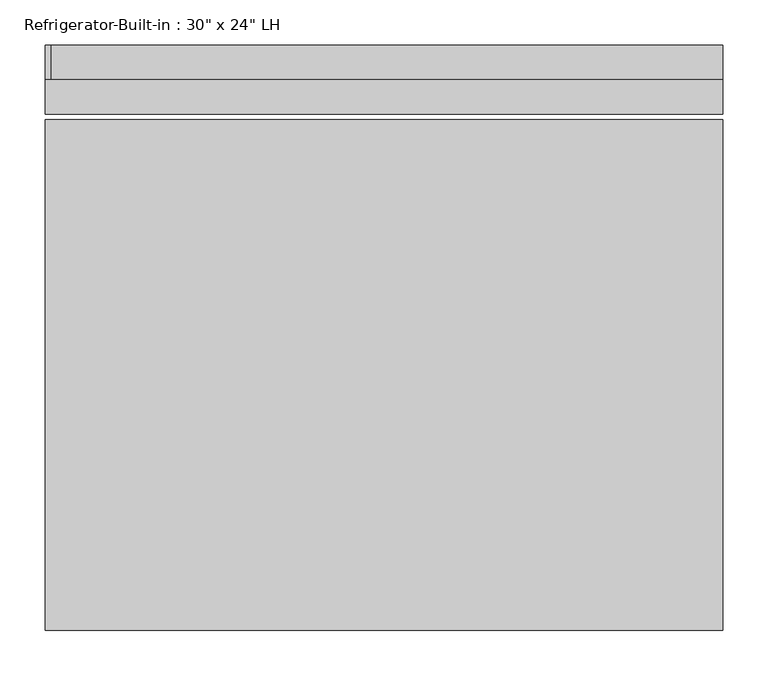
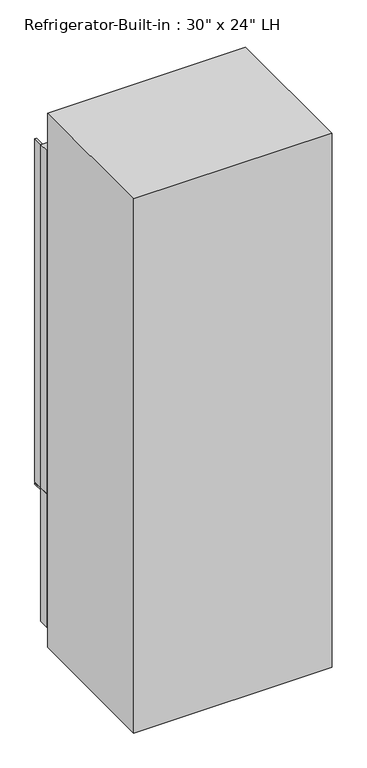
"""IFC4 building model written with IfcOpenShell, lengths in millimetres: proxy geometry."""

from ifc_helpers import new_model, si_unit, frame, origin, origin_with_axes, place, context, project, spatial, polyline, outline, extrude, source, transform, mapped, element, save


def proxy_76352e5b(model_context):
    return source(origin(), model_context, "Body", "SweptSolid", [
        extrude(outline(polyline([(374.65, -290.1239715), (-374.65, -290.1239715), (-374.65, 275.0260285), (374.65, 275.0260285), (374.65, -290.1239715)])), origin_with_axes(), (0.0, 0.0, 1.0), 2133.6),
        extrude(outline(polyline([(374.65, 281.3760285), (-374.65, 281.3760285), (-374.65, 319.4760285), (374.65, 319.4760285), (374.65, 281.3760285)])), frame((0.0, 0.0, 611.1875), z_axis=(0.0, 0.0, 1.0), x_axis=(1.0, 0.0, 0.0)), (0.0, 0.0, 1.0), 1370.0125),
        extrude(outline(polyline([(374.65, 281.3760285), (-374.65, 281.3760285), (-374.65, 319.4760285), (374.65, 319.4760285), (374.65, 281.3760285)])), frame((0.0, 0.0, 76.2), z_axis=(0.0, 0.0, 1.0), x_axis=(1.0, 0.0, 0.0)), (0.0, 0.0, 1.0), 531.8125),
        extrude(outline(polyline([(374.65, 319.4760285), (-374.65, 319.4760285), (-374.65, 357.5760285), (374.65, 357.5760285), (374.65, 319.4760285)])), frame((0.0, 0.0, 601.6625), z_axis=(0.0, 0.0, 1.0), x_axis=(1.0, 0.0, 0.0)), (0.0, 0.0, 1.0), 6.35),
        extrude(outline(polyline([(-374.65, 319.4760285), (-374.65, 357.5760285), (-368.3, 357.5760285), (-368.3, 319.4760285), (-374.65, 319.4760285)])), frame((0.0, 0.0, 611.1875), z_axis=(0.0, 0.0, 1.0), x_axis=(1.0, 0.0, 0.0)), (0.0, 0.0, 1.0), 1370.0125),
    ])


if __name__ == "__main__":
    model = new_model("IFC4")
    model_context = context("Model", 3, world=origin())
    ifc_project = project(units=[si_unit("LENGTHUNIT", "METRE", prefix="MILLI")], contexts=[model_context])
    site = spatial("IfcSite", under=ifc_project)
    building = spatial("IfcBuilding", under=site)
    placement = place(None, origin())
    proxy_shape = proxy_76352e5b(model_context)
    element("IfcBuildingElementProxy", 1, Name="Refrigerator-Built-in : 30\" x 24\" LH", ObjectType="Refrigerator-Built-in : 30\" x 24\" LH", at=placement, inside=building, context=model_context, shape_type="MappedRepresentation", body=[
        mapped(proxy_shape, transform((0.0, 0.0, 0.0), x_axis=(1.0, 0.0, 0.0), y_axis=(0.0, 1.0, 0.0), z_axis=(0.0, 0.0, 1.0))),
    ])
    save(model, "model.ifc")

# Revit data of these elements
# Type "Refrigerator-Built-in : 30\" x 24\" LH"
#   Assembly Code = "E1090400"
#   Depth = 2' - 0"
#   Handle = 0' - 0 1/4"
#   Height = 7' - 0"
#   Top Door Height = 5' - 0"
#   Width = 2' - 5 1/2"
#   Material = Metal - Paint Finish - Ivory,Glossy
#   Default Elevation = 0
# Element 1 (IfcBuildingElementProxy, "Refrigerator-Built-in : 30\" x 24\" LH")
#   Materials on its faces: "Metal - Paint Finish - Ivory,Glossy", "Metal - Chrome"
# Materials
#   "Metal - Paint Finish - Ivory,Glossy": colour RGB 247 247 239, transparency 0
#   "Metal - Chrome": colour RGB 17 17 17, transparency 0
